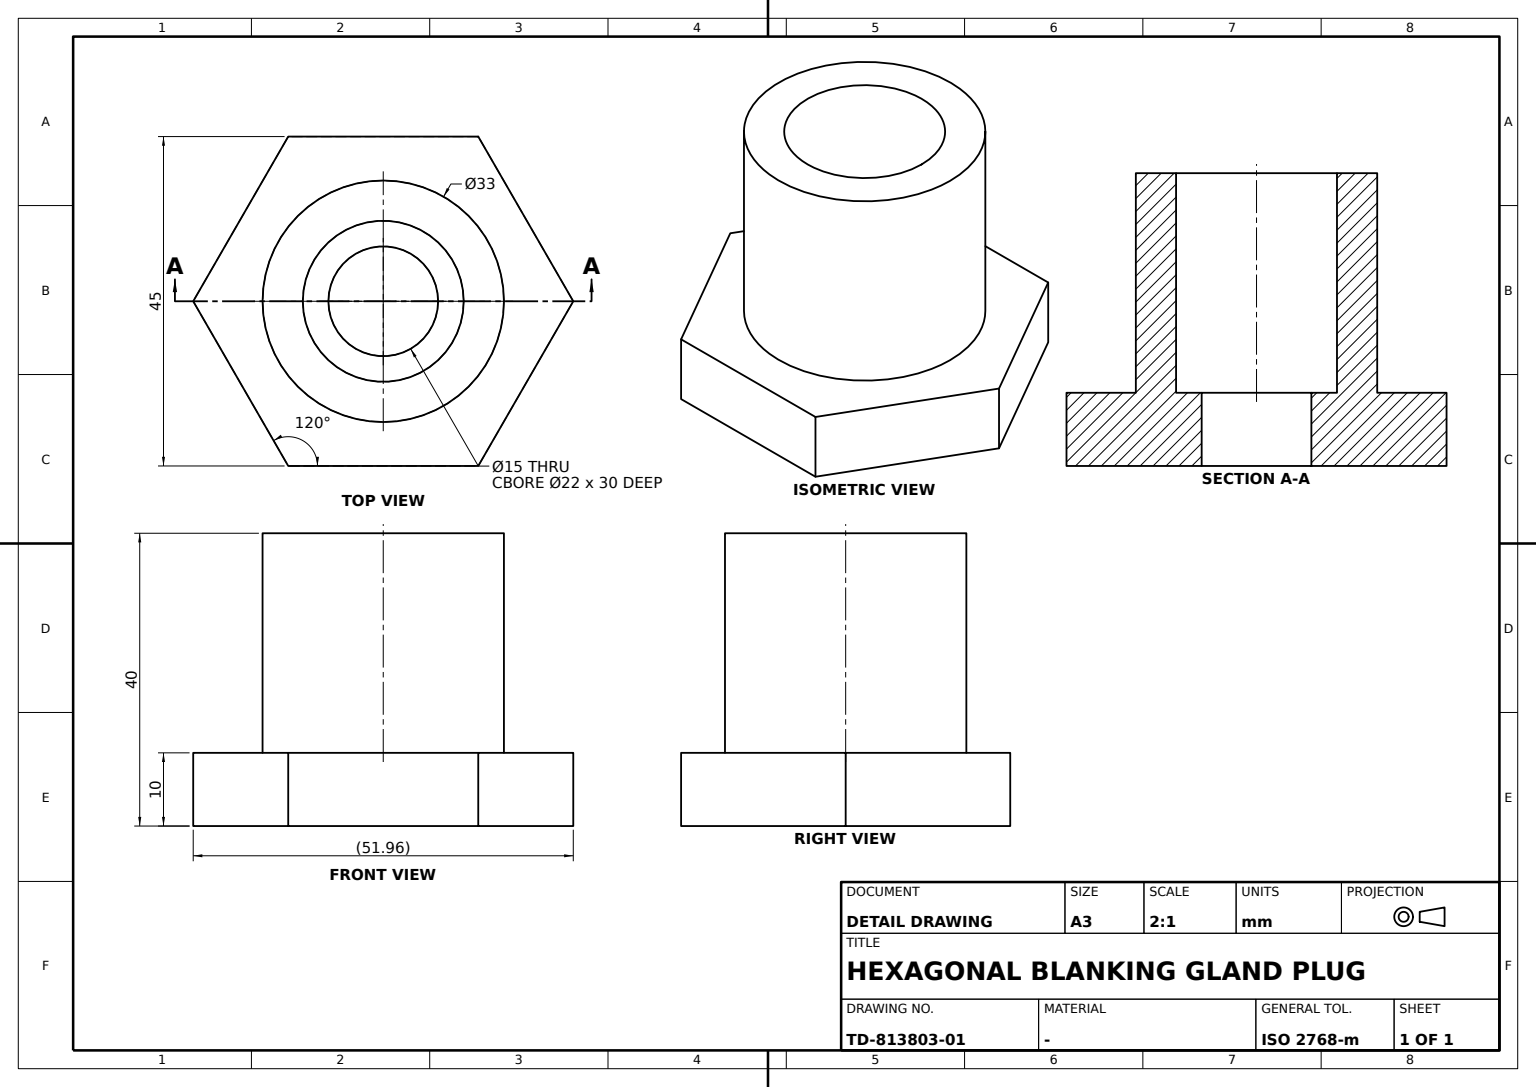
CATIA V5 part; units mm, degrees
sketch "Sketch1" plane through (0, 0, 0) normal (0, 0, 1) x (1, 0, 0)
  point P0 (12.9904, 22.5)
  point P1 (-12.9904, 22.5)
  point P2 (-25.9808, 0)
  point P3 (-12.9904, -22.5)
  point P4 (12.9904, -22.5)
  point P5 (25.9808, 0)
  point P6 (0, 22.5)
  line L0 (12.9904, 22.5) -> (-12.9904, 22.5)
  line L1 (-12.9904, 22.5) -> (-25.9808, 0)
  line L2 (-25.9808, 0) -> (-12.9904, -22.5)
  line L3 (-12.9904, -22.5) -> (12.9904, -22.5)
  line L4 (12.9904, -22.5) -> (25.9808, 0)
  line L5 (25.9808, 0) -> (12.9904, 22.5)
  line L6 (0, 0) -> (0, 22.5) construction
  circle A0 centre (0, 0) radius 25.9808 construction
  arc A1 (-12.9904, -22.5) -> (25.9808, 0) centre (12.9904, -22.5) cw construction
  arc A2 (-25.9808, 0) -> (12.9904, 22.5) centre (-12.9904, 22.5) ccw construction
  dimension "distance L0 L3" = 45
  constraint coincidence A0 P0
  constraint coincidence A0 P1
  constraint coincidence A0 P2
  constraint coincidence A0 P3
  constraint coincidence A0 P4
  constraint coincidence A0 P5
  constraint coincidence A1 origin
  constraint coincidence A2 origin
  constraint midpoint P6 L0
extrude "Pad1" add sketch "Sketch1" along normal blind 10
sketch "Sketch2" plane through (0, 0, 10) normal (0, 0, 1) x (1, 0, 0)
  circle A0 centre (0, 0) radius 16.5
  circle A1 centre (0, 0) radius 11
  dimension "radius A0" = 16.5
  dimension "radius A1" = 11
extrude "Pad2" add sketch "Sketch2" along normal blind 30
sketch "Sketch3" plane through (0, 0, 10) normal (0, 0, 1) x (1, 0, 0)
  circle A0 centre (0, 0) radius 7.5
  dimension "radius A0" = 7.5
extrude "Pocket1" cut sketch "Sketch3" against normal blind 30
